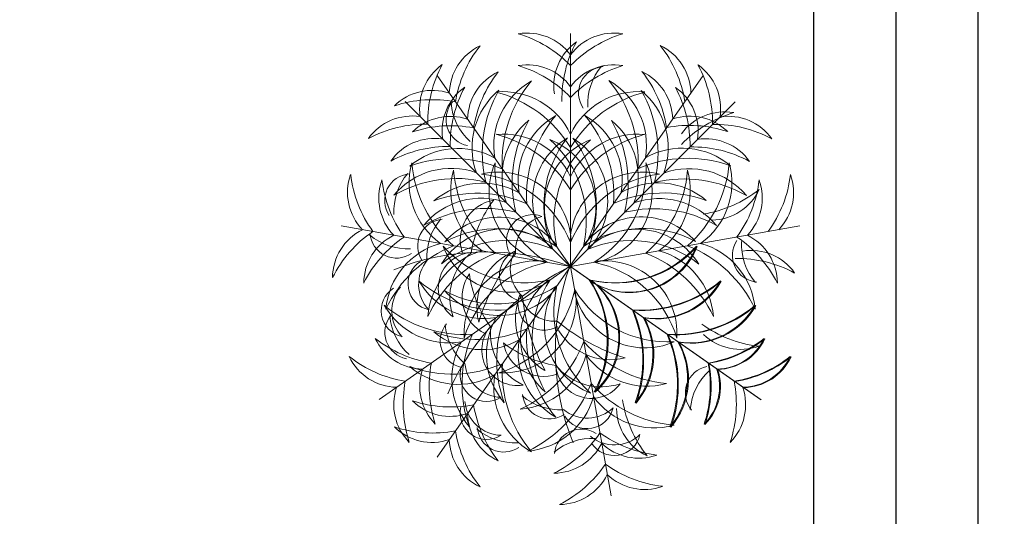
# Model space of a CAD drawing. Units: inches. Extents: x -48 to 50072, y 0 to 21068.
# Tile 38 of 75: x 501 to 555, y 279 to 306. Entities that reach past the tile are written whole.
import ezdxf

# ---------------------------------------------------------------- set-up
doc = ezdxf.new("R2010")
doc.units = ezdxf.units.IN
doc.header["$MEASUREMENT"] = 0
doc.linetypes.add('ACAD_ISO02W100', pattern=[15, 12, -3])
for name, color, linetype, lineweight in [('A-ANNO-DIMS', 2, 'Continuous', 18), ('C-PROP', 7, 'Continuous', 25), ('C-PROP-REF', 32, 'ACAD_ISO02W100', 13), ('L-PLNT', 94, 'Continuous', 13)]:
    doc.layers.add(name, color=color, linetype=linetype, lineweight=lineweight)
doc.styles.get("Standard").update_dxf_attribs({"font": 'arial.ttf'})
doc.dimstyles.get("Standard").update_dxf_attribs({"dimtxt": 8, "dimasz": 0.18, "dimexe": 0.18, "dimexo": 0.0625, "dimgap": 0.09, "dimtad": 0, "dimtih": 1, "dimtoh": 1, "dimdec": 1, "dimzin": 0, "dimdsep": 46, "dimlunit": 4, "dimtxsty": 'Standard', "dimblk": 'ARCHTICK', "dimcen": 0.09, "dimadec": 0, "dimazin": 0, "dimtfac": 1, "dimtdec": 1, "dimtofl": 0, "dimtmove": 0, "dimatfit": 3, "dimldrblk": 'ARCHTICK', "dimfxl": 1, "dimtolj": 1, "dimtzin": 0, "dimarcsym": 0})

# ---------------------------------------------------------------- blocks, each defined once
blk = doc.blocks.new('A$C5D061C3B')
for p, q in [((3.377, 6.679), (3.377, 3.377)), ((1.483, 6.082), (3.377, 3.377)), ((5.259, 6.086), (3.365, 3.381)), ((1.03, 5.716), (3.365, 3.381)), ((5.712, 5.712), (3.377, 3.377)), ((0.125, 3.951), (3.377, 3.377)), ((6.629, 3.951), (3.377, 3.377)), ((0.66, 1.487), (3.365, 3.381)), ((1.483, 0.672), (3.377, 3.377)), ((6.07, 1.487), (3.365, 3.381)), ((3.951, 0.125), (3.377, 3.377)), ((6.082, 1.483), (3.377, 3.377))]:
    blk.add_line(p, q)
for centre, radius, start, end in [((2.763, 5.924), 0.762, 36.29, 99.6243), ((2.145, 5.032), 1.715, 44.0763, 73.3794), ((3.991, 5.924), 0.762, 80.3757, 143.71), ((4.61, 5.032), 1.715, 106.6206, 135.9237), ((2.419, 5.816), 0.762, 115.3757, 178.71), ((3.438, 5.44), 1.715, 141.6206, 170.9237), ((3.901, 5.939), 0.762, 125.3757, 188.71), ((4.969, 5.745), 1.715, 151.6206, 180.9237), ((3.305, 5.444), 1.715, 9.0763, 38.3794), ((4.323, 5.82), 0.762, 1.29, 64.6243), ((1.998, 5.617), 0.762, 125.3757, 188.71), ((3.066, 5.423), 1.715, 151.6206, 180.9237), ((2.763, 5.474), 0.762, 36.29, 99.6243), ((2.145, 4.581), 1.715, 44.0763, 73.3794), ((3.991, 5.474), 0.762, 80.3757, 143.71), ((4.61, 4.581), 1.715, 106.6206, 135.9237), ((3.871, 5.832), 0.38, 94.742, 213.7475), ((4.447, 5.681), 0.826, 139.618, 183.2106), ((4.744, 5.613), 0.762, 351.29, 54.6243), ((3.676, 5.419), 1.715, 359.0763, 28.3794), ((2.678, 5.447), 0.762, 115.3757, 178.71), ((3.696, 5.07), 1.715, 141.6206, 170.9237), ((3.344, 5.089), 1.056, 119.6063, 189.7511), ((4.177, 4.869), 1.77, 139.9634, 183.6288), ((3.398, 5.094), 1.056, 350.2489, 60.3937), ((2.565, 4.873), 1.77, 356.3712, 40.0366), ((4.064, 5.451), 0.762, 1.29, 64.6243), ((3.046, 5.075), 1.715, 9.0763, 38.3794), ((1.413, 5.111), 0.762, 71.29, 134.6243), ((2.317, 5.298), 0.762, 125.3757, 188.71), ((3.385, 5.104), 1.715, 151.6206, 180.9237), ((3.035, 5.062), 1.056, 129.6063, 199.7511), ((3.894, 4.989), 1.77, 149.9634, 193.6288), ((2.848, 4.985), 1.77, 346.3712, 30.0366), ((3.707, 5.058), 1.056, 340.2489, 50.3937), ((3.357, 5.1), 1.715, 359.0763, 28.3794), ((4.425, 5.294), 0.762, 351.29, 54.6243), ((1.419, 4.026), 1.715, 79.0763, 108.3794), ((2.422, 4.799), 1.056, 25.2489, 95.3937), ((1.866, 4.14), 1.77, 31.3712, 75.0366), ((4.332, 4.799), 1.056, 84.6063, 154.7511), ((4.888, 4.14), 1.77, 104.9634, 148.6288), ((1.991, 5.462), 0.38, 139.742, 258.7475), ((2.505, 5.763), 0.826, 184.618, 228.2106), ((1.13, 4.748), 0.762, 81.29, 144.6243), ((1.671, 4.742), 0.762, 71.29, 134.6243), ((3.46, 4.637), 1.056, 129.6063, 199.7511), ((4.319, 4.565), 1.77, 149.9634, 193.6288), ((3.688, 4.597), 1.056, 119.6063, 189.7511), ((4.522, 4.377), 1.77, 139.9634, 183.6288), ((2.221, 4.381), 1.77, 356.3712, 40.0366), ((3.054, 4.602), 1.056, 350.2489, 60.3937), ((5.071, 4.746), 0.762, 45.3757, 108.71), ((5.564, 4.807), 0.762, 80.3757, 143.71), ((6.182, 3.914), 1.715, 106.6206, 135.9237), ((5.613, 4.744), 0.762, 35.3757, 98.71), ((1.324, 3.68), 1.715, 89.0763, 118.3794), ((1.677, 3.657), 1.715, 79.0763, 108.3794), ((3.283, 4.633), 1.056, 340.2489, 50.3937), ((2.424, 4.56), 1.77, 346.3712, 30.0366), ((5.065, 3.661), 1.715, 71.6206, 100.9237), ((5.419, 3.676), 1.715, 61.6206, 90.9237), ((1.448, 4.43), 0.762, 81.29, 144.6243), ((2.422, 4.198), 1.056, 25.2489, 95.3937), ((1.866, 3.54), 1.77, 31.3712, 75.0366), ((3.868, 4.321), 1.029, 121.3654, 221.5741), ((4.556, 4.237), 1.557, 141.8122, 203.3335), ((4.035, 4.215), 1.029, 111.3654, 211.5741), ((2.707, 4.219), 1.029, 328.4259, 68.6346), ((2.044, 4.017), 1.557, 346.6665, 48.1878), ((4.698, 4.013), 1.557, 131.8122, 193.3335), ((4.332, 4.198), 1.056, 84.6063, 154.7511), ((4.888, 3.54), 1.77, 104.9634, 148.6288), ((2.187, 4.233), 1.557, 336.6665, 38.1878), ((2.875, 4.316), 1.029, 318.4259, 58.6346), ((5.294, 4.425), 0.762, 35.3757, 98.71), ((1.642, 3.362), 1.715, 89.0763, 118.3794), ((1.78, 3.994), 1.056, 60.2489, 130.3937), ((4.963, 3.998), 1.056, 49.6063, 119.7511), ((5.1, 3.357), 1.715, 61.6206, 90.9237), ((1.702, 3.136), 1.77, 66.3712, 110.0366), ((5.04, 3.14), 1.77, 69.9634, 113.6288), ((1.685, 3.712), 1.056, 70.2489, 140.3937), ((2.143, 4.564), 1.056, 164.6063, 234.7511), ((2.888, 4.998), 1.77, 184.9634, 228.6288), ((3.25, 4.435), 1.029, 156.3654, 256.5741), ((3.862, 4.761), 1.557, 176.8122, 238.3335), ((2.893, 4.761), 1.557, 301.6665, 3.1878), ((3.504, 4.435), 1.029, 283.4259, 23.6346), ((5.058, 3.707), 1.056, 39.6063, 109.7511), ((3.866, 4.998), 1.77, 311.3712, 355.0366), ((4.611, 4.564), 1.056, 305.2489, 15.3937), ((0.975, 4.424), 0.762, 160.3757, 223.71), ((1.962, 4.878), 1.715, 186.6206, 215.9237), ((1.12, 4.31), 0.38, 94.742, 213.7475), ((1.696, 4.159), 0.826, 139.618, 183.2106), ((1.757, 2.853), 1.77, 76.3712, 120.0366), ((2.734, 4.46), 1.056, 164.6063, 234.7511), ((3.48, 4.893), 1.77, 184.9634, 228.6288), ((2.358, 3.686), 1.029, 3.4259, 103.6346), ((1.93, 3.14), 1.557, 21.6665, 83.1878), ((4.397, 3.686), 1.029, 76.3654, 176.5741), ((4.824, 3.14), 1.557, 96.8122, 158.3335), ((3.275, 4.893), 1.77, 311.3712, 355.0366), ((4.985, 2.848), 1.77, 59.9634, 103.6288), ((4.02, 4.46), 1.056, 305.2489, 15.3937), ((4.793, 4.878), 1.715, 324.0763, 353.3794), ((5.779, 4.424), 0.762, 316.29, 19.6243), ((1.419, 4.346), 0.762, 160.3757, 223.71), ((2.405, 4.8), 1.715, 186.6206, 215.9237), ((2.124, 3.502), 1.056, 60.2489, 130.3937), ((4.618, 3.506), 1.056, 49.6063, 119.7511), ((4.349, 4.8), 1.715, 324.0763, 353.3794), ((5.335, 4.346), 0.762, 316.29, 19.6243), ((2.109, 3.287), 1.056, 70.2489, 140.3937), ((2.046, 2.644), 1.77, 66.3712, 110.0366), ((4.696, 2.648), 1.77, 69.9634, 113.6288), ((4.633, 3.283), 1.056, 39.6063, 109.7511), ((4.988, 5.812), 1.715, 279.0763, 308.3794), ((5.365, 4.794), 0.762, 271.29, 334.6243), ((2.182, 2.428), 1.77, 76.3712, 120.0366), ((2.387, 3.752), 0.574, 99.9865, 199.4034), ((3.599, 3.314), 1.651, 142.5759, 170.8942), ((4.56, 2.424), 1.77, 59.9634, 103.6288), ((2.365, 3.045), 1.029, 38.4259, 138.6346), ((2.84, 3.739), 0.372, 69.2257, 210.1279), ((3.109, 3.59), 0.515, 105.4398, 183.6694), ((4.377, 3.05), 1.029, 41.3654, 141.5741), ((1.588, 3.666), 0.38, 94.742, 213.7475), ((2.165, 3.515), 0.826, 139.618, 183.2106), ((4.414, 2.358), 1.557, 61.8122, 123.3335), ((0.762, 3.214), 0.762, 116.29, 179.6243), ((1.534, 2.451), 1.715, 124.0763, 153.3794), ((1.206, 3.136), 0.762, 116.29, 179.6243), ((1.977, 2.373), 1.715, 124.0763, 153.3794), ((1.062, 4.452), 0.826, 229.618, 273.2106), ((0.91, 3.875), 0.38, 184.742, 303.7475), ((2.426, 2.879), 1.029, 48.4259, 148.6346), ((2.328, 2.353), 1.557, 56.6665, 118.1878), ((4.316, 2.875), 1.029, 31.3654, 131.5741), ((4.777, 2.373), 1.715, 26.6206, 55.9237), ((5.549, 3.136), 0.762, 0.3757, 63.71), ((1.811, 2.684), 1.056, 105.2489, 175.3937), ((2.363, 2.022), 1.77, 111.3712, 155.0366), ((2.51, 2.191), 1.557, 66.6665, 128.1878), ((2.729, 4.702), 1.557, 221.8122, 283.3335), ((2.527, 4.039), 1.029, 201.3654, 301.5741), ((4.233, 2.187), 1.557, 51.8122, 113.3335), ((4.001, 4.702), 1.557, 256.6665, 318.1878), ((4.013, 4.698), 1.557, 256.6665, 318.1878), ((4.203, 4.039), 1.029, 238.4259, 338.6346), ((4.215, 4.035), 1.029, 238.4259, 338.6346), ((4.391, 2.022), 1.77, 24.9634, 68.6288), ((4.943, 2.684), 1.056, 4.6063, 74.7511), ((6.053, 3.533), 0.38, 146.2525, 265.258), ((6.629, 3.684), 0.826, 176.7894, 220.382), ((2.185, 0.015), 3.567, 70.4772, 111.6585), ((2.403, 2.58), 1.056, 105.2489, 175.3937), ((2.955, 1.917), 1.77, 111.3712, 155.0366), ((2.007, 3.071), 0.506, 93.8744, 233.9763), ((2.489, 2.932), 0.825, 128.7536, 199.097), ((2.903, 2.8), 0.855, 116.4477, 194.3672), ((4.744, 1.779), 2.789, 140.4007, 163.139), ((2.741, 3.253), 0.372, 114.2257, 255.1279), ((3.037, 3.338), 0.515, 150.4398, 228.6694), ((3.799, 1.917), 1.77, 24.9634, 68.6288), ((4.352, 2.58), 1.056, 4.6063, 74.7511), ((5.935, 2.842), 0.762, 35.3757, 98.71), ((1.447, 3.129), 0.376, 122.0577, 257.8533), ((1.751, 3.126), 0.529, 140.1845, 223.654), ((4.912, 0.157), 3.567, 115.4772, 156.6585), ((2.896, 2.427), 1.029, 83.4259, 183.6346), ((3.359, 1.911), 1.557, 101.6665, 163.1878), ((6.727, 2.189), 3.567, 160.4772, 201.6585), ((3.395, 1.911), 1.557, 16.8122, 78.3335), ((3.858, 2.427), 1.029, 356.3654, 96.5741), ((5.741, 1.774), 1.715, 61.6206, 90.9237), ((2.412, 2.943), 0.574, 144.9865, 244.4034), ((3.578, 3.49), 1.651, 187.5759, 215.8942), ((1.37, 2.745), 0.529, 140.1845, 223.654), ((2.145, 3.693), 1.056, 209.6063, 279.7511), ((2.365, 4.526), 1.77, 229.9634, 273.6288), ((2.328, 4.401), 1.557, 241.8122, 303.3335), ((3.697, 2.369), 1.029, 128.4259, 228.6346), ((4.389, 2.332), 1.557, 146.6665, 208.1878), ((4.035, 2.539), 1.029, 148.4259, 248.6346), ((4.698, 2.741), 1.557, 166.6665, 228.1878), ((2.341, 2.332), 1.557, 331.8122, 33.3335), ((2.353, 2.328), 1.557, 331.8122, 33.3335), ((3.033, 2.369), 1.029, 311.3654, 51.5741), ((3.045, 2.365), 1.029, 311.3654, 51.5741), ((4.365, 4.526), 1.77, 266.3712, 310.0366), ((4.377, 4.522), 1.77, 266.3712, 310.0366), ((4.585, 3.693), 1.056, 260.2489, 330.3937), ((4.597, 3.688), 1.056, 260.2489, 330.3937), ((1.067, 2.749), 0.376, 122.0577, 257.8533), ((2.365, 3.709), 1.029, 221.3654, 321.5741), ((1.911, 3.359), 1.557, 286.8122, 348.3335), ((2.427, 2.896), 1.029, 266.3654, 6.5741), ((3.003, 2.844), 0.372, 159.2257, 300.1279), ((3.152, 3.113), 0.515, 195.4398, 273.6694), ((5.474, 3.214), 2.789, 185.4007, 208.139), ((4.435, 3.25), 1.029, 193.4259, 293.6346), ((4.761, 3.862), 1.557, 211.6665, 273.1878), ((1.873, 4.181), 1.77, 229.9634, 273.6288), ((1.653, 3.348), 1.056, 209.6063, 279.7511), ((3.45, 2.634), 0.855, 161.4477, 239.3672), ((4.857, 4.181), 1.77, 266.3712, 310.0366), ((4.869, 4.177), 1.77, 266.3712, 310.0366), ((5.077, 3.348), 1.056, 260.2489, 330.3937), ((5.089, 3.344), 1.056, 260.2489, 330.3937), ((1.122, 2.441), 0.38, 139.742, 258.7475), ((1.636, 2.741), 0.826, 184.618, 228.2106), ((4.099, 2.051), 1.77, 156.3712, 200.0366), ((2.632, 2.051), 1.77, 339.9634, 23.6288), ((2.644, 2.046), 1.77, 339.9634, 23.6288), ((1.908, 2.317), 0.38, 139.742, 258.7475), ((2.422, 2.617), 0.826, 184.618, 228.2106), ((2.624, 2.192), 0.506, 138.8744, 278.9763), ((3.24, 2.128), 1.056, 150.2489, 220.3937), ((3.064, 2.435), 0.825, 173.7536, 244.097), ((3.942, 2.908), 0.855, 206.4477, 284.3672), ((4.963, 4.749), 2.789, 230.4007, 253.139), ((3.49, 2.128), 1.056, 319.6063, 29.7511), ((3.502, 2.124), 1.056, 319.6063, 29.7511), ((6.244, 3.948), 1.715, 234.0763, 263.3794), ((2.046, 4.111), 1.77, 249.9634, 293.6288), ((2.124, 3.252), 1.056, 229.6063, 299.7511), ((3.607, 1.706), 1.77, 156.3712, 200.0366), ((4.522, 2.378), 1.77, 176.3712, 220.0366), ((3.124, 1.706), 1.77, 339.9634, 23.6288), ((3.136, 1.702), 1.77, 339.9634, 23.6288), ((5.79, 2.962), 0.762, 226.29, 289.6243), ((1.672, 3.7), 1.715, 231.6206, 260.9237), ((1.295, 2.682), 0.762, 205.3757, 268.71), ((2.748, 1.784), 1.056, 150.2489, 220.3937), ((3.428, 3.603), 1.651, 232.5759, 260.8942), ((2.99, 2.391), 0.574, 189.9865, 289.4034), ((3.688, 2.157), 1.056, 170.2489, 240.3937), ((1.917, 2.955), 1.77, 294.9634, 338.6288), ((4.893, 3.48), 1.77, 221.3712, 265.0366), ((3.982, 1.784), 1.056, 319.6063, 29.7511), ((3.994, 1.78), 1.056, 319.6063, 29.7511), ((5.058, 3.7), 1.715, 279.0763, 308.3794), ((5.07, 3.696), 1.715, 279.0763, 308.3794), ((5.435, 2.682), 0.762, 271.29, 334.6243), ((5.447, 2.678), 0.762, 271.29, 334.6243), ((0.926, 2.424), 0.762, 205.3757, 268.71), ((1.303, 3.442), 1.715, 231.6206, 260.9237), ((2.58, 2.403), 1.056, 274.6063, 344.7511), ((4.46, 2.734), 1.056, 215.2489, 285.3937), ((5.427, 3.442), 1.715, 279.0763, 308.3794), ((5.804, 2.424), 0.762, 271.29, 334.6243), ((1.702, 3.619), 1.77, 249.9634, 293.6288), ((1.78, 2.76), 1.056, 229.6063, 299.7511), ((3.086, 1.681), 1.715, 169.0763, 198.3794), ((2.405, 2.049), 0.529, 185.1845, 268.654), ((4.177, 1.886), 1.77, 176.3712, 220.0366), ((3.81, 2.493), 0.825, 218.7536, 289.097), ((3.671, 2.011), 0.506, 183.8744, 323.9763), ((5.385, 1.584), 0.38, 101.2525, 220.258), ((3.645, 1.681), 1.715, 341.6206, 10.9237), ((3.657, 1.677), 1.715, 341.6206, 10.9237), ((5.44, 3.438), 1.715, 279.0763, 308.3794), ((5.816, 2.419), 0.762, 271.29, 334.6243), ((2, 1.676), 0.762, 161.29, 224.6243), ((2.188, 1.837), 0.376, 167.0577, 302.8533), ((3.344, 1.665), 1.056, 170.2489, 240.3937), ((5.899, 1.283), 0.826, 131.7894, 175.382), ((4.73, 1.676), 0.762, 315.3757, 18.71), ((4.742, 1.671), 0.762, 315.3757, 18.71), ((2.717, 1.423), 1.715, 169.0763, 198.3794), ((2.022, 2.363), 1.77, 294.9634, 338.6288), ((4.998, 2.888), 1.77, 221.3712, 265.0366), ((4.014, 1.423), 1.715, 341.6206, 10.9237), ((1.631, 1.417), 0.762, 161.29, 224.6243), ((3.227, 2.169), 0.826, 229.618, 273.2106), ((3.076, 1.593), 0.38, 184.742, 303.7475), ((5.099, 1.417), 0.762, 315.3757, 18.71), ((1.671, 2.012), 0.762, 225.3757, 288.71), ((1.677, 3.098), 1.715, 251.6206, 280.9237), ((2.405, 1.511), 0.529, 185.1845, 268.654), ((3.696, 1.684), 1.715, 189.0763, 218.3794), ((2.684, 1.811), 1.056, 274.6063, 344.7511), ((4.564, 2.143), 1.056, 215.2489, 285.3937), ((5.808, 1.754), 1.715, 189.0763, 218.3794), ((2.188, 1.299), 0.376, 167.0577, 302.8533), ((2.678, 1.307), 0.762, 181.29, 244.6243), ((3.616, 1.755), 0.529, 230.1845, 313.654), ((3.613, 1.452), 0.376, 212.0577, 347.8533), ((4.79, 1.377), 0.762, 181.29, 244.6243), ((1.419, 2.729), 1.715, 251.6206, 280.9237), ((1.413, 1.643), 0.762, 225.3757, 288.71), ((3.438, 1.315), 1.715, 189.0763, 218.3794), ((2.583, 1.701), 0.826, 229.618, 273.2106), ((2.432, 1.124), 0.38, 184.742, 303.7475), ((2.373, 1.977), 1.715, 296.6206, 325.9237), ((3.528, 0.69), 0.38, 56.2525, 175.258), ((3.997, 1.374), 0.529, 230.1845, 313.654), ((3.994, 1.071), 0.376, 212.0577, 347.8533), ((4.8, 2.405), 1.715, 234.0763, 263.3794), ((2.419, 0.938), 0.762, 181.29, 244.6243), ((3.136, 1.206), 0.762, 270.3757, 333.71), ((3.68, 0.113), 0.826, 86.7894, 130.382), ((4.346, 1.419), 0.762, 226.29, 289.6243), ((2.451, 1.534), 1.715, 296.6206, 325.9237), ((4.878, 1.962), 1.715, 234.0763, 263.3794), ((3.214, 0.762), 0.762, 270.3757, 333.71), ((4.424, 0.975), 0.762, 226.29, 289.6243)]:
    blk.add_arc(centre, radius, start, end)
blk = doc.blocks.new('_ArchTick')
at = {"color": 0, "linetype": 'ByBlock', "const_width": 0.15}
blk.add_lwpolyline([(-0.5, -0.5), (0.5, 0.5)], dxfattribs=at)
blk = doc.blocks.new('*D54')
at = {"layer": 'A-ANNO-DIMS', "color": 0, "lineweight": -2, "transparency": 16777216}
for p, q in [((540.551, 275.597), (544.198, 275.597)), ((544.018, 275.597), (544.018, 268.06)), ((544.018, 252.07), (544.018, 259.607)), ((540.551, 252.07), (544.198, 252.07))]:
    blk.add_line(p, q, dxfattribs=at)
at = {"layer": 'Defpoints', "color": 0, "transparency": 16777216}
for p in [(540.489, 275.597), (544.018, 275.597), (540.489, 252.07)]:
    blk.add_point(p, dxfattribs=at)
at = {"layer": 'A-ANNO-DIMS', "color": 0, "lineweight": -2, "transparency": 16777216, "xscale": 0.18, "yscale": 0.18, "zscale": 0.18}
for p, rotation in [((544.018, 275.597), 90), ((544.018, 252.07), 270)]:
    blk.add_blockref('_ArchTick', p, dxfattribs=dict(at, rotation=rotation))
at = {"layer": 'A-ANNO-DIMS', "color": 0, "transparency": 16777216, "insert": (544.018, 263.834), "char_height": 8, "attachment_point": 5}
blk.add_mtext('\\A1;SHRUB B 24 TYP.', dxfattribs=at)
blk = doc.blocks.new('*D115')
at = {"layer": 'A-ANNO-DIMS', "color": 0, "lineweight": -2, "transparency": 16777216}
for p, q in [((549.08, 451.075), (601.647, 451.075)), ((601.467, 451.075), (601.467, 336.752)), ((601.467, 214.075), (601.467, 328.397)), ((553.58, 214.075), (601.647, 214.075))]:
    blk.add_line(p, q, dxfattribs=at)
at = {"layer": 'Defpoints', "color": 0, "transparency": 16777216}
for p in [(549.017, 451.075), (601.467, 451.075), (553.517, 214.075)]:
    blk.add_point(p, dxfattribs=at)
at = {"layer": 'A-ANNO-DIMS', "color": 0, "lineweight": -2, "transparency": 16777216, "xscale": 0.18, "yscale": 0.18, "zscale": 0.18}
for p, rotation in [((601.467, 451.075), 90), ((601.467, 214.075), 270)]:
    blk.add_blockref('_ArchTick', p, dxfattribs=dict(at, rotation=rotation))
at = {"layer": 'A-ANNO-DIMS', "color": 0, "transparency": 16777216, "insert": (601.467, 332.575), "char_height": 8, "attachment_point": 5}
blk.add_mtext('\\A1;237', dxfattribs=at)
blk = doc.blocks.new('*D119')
at = {"layer": 'A-ANNO-DIMS', "color": 0, "lineweight": -2, "transparency": 16777216}
for p, q in [((463.517, 451.012), (463.517, 165.945)), ((549.017, 451.012), (549.017, 165.945)), ((463.517, 166.125), (495.752, 166.125)), ((549.017, 166.125), (516.783, 166.125))]:
    blk.add_line(p, q, dxfattribs=at)
at = {"layer": 'Defpoints', "color": 0, "transparency": 16777216}
for p in [(463.517, 451.075), (549.017, 451.075), (549.017, 166.125)]:
    blk.add_point(p, dxfattribs=at)
at = {"layer": 'A-ANNO-DIMS', "color": 0, "lineweight": -2, "transparency": 16777216, "xscale": 0.18, "yscale": 0.18, "zscale": 0.18, "rotation": 180}
blk.add_blockref('_ArchTick', (463.517, 166.125), dxfattribs=at)
at = {"layer": 'A-ANNO-DIMS', "color": 0, "lineweight": -2, "transparency": 16777216, "xscale": 0.18, "yscale": 0.18, "zscale": 0.18}
blk.add_blockref('_ArchTick', (549.017, 166.125), dxfattribs=at)
at = {"layer": 'A-ANNO-DIMS', "color": 0, "transparency": 16777216, "insert": (506.267, 166.125), "char_height": 8, "attachment_point": 5}
blk.add_mtext('\\A1;85.5', dxfattribs=at)

msp = doc.modelspace()

# ---------------------------------------------------------------- linework, layer by layer
at = {"layer": 'C-PROP'}
for p, q in [((553.517, 214.075), (553.517, 1170.775)), ((544.517, 223.075), (544.517, 488.775))]:
    msp.add_line(p, q, dxfattribs=at)
at = {"layer": 'C-PROP-REF'}
msp.add_line((549.017, 214.075), (549.017, 1166.275), dxfattribs=at)

# ---------------------------------------------------------------- block references
at = {"layer": 'L-PLNT', "xscale": 3.862191520948588, "yscale": 3.862191520948588, "zscale": 3.862191520948588}
msp.add_blockref('A$C5D061C3B', (518.144, 279.329), dxfattribs=at)

# ---------------------------------------------------------------- dimensions: what is measured, and where the dimension line sits
at = {"layer": 'A-ANNO-DIMS'}
dim = msp.add_linear_dim(base=(549.017, 166.125), p1=(463.517, 451.075), p2=(549.017, 451.075), dimstyle='Standard', override={"dimdec": 1, "dimlfac": 1, "dimrnd": 0, "dimzin": 0, "dimdsep": 46, "dimlunit": 2}, dxfattribs=at)
dim.commit()
dim.dimension.update_dxf_attribs({"geometry": '*D119', "text_midpoint": (506.267, 166.125)})
dim = msp.add_linear_dim(base=(601.467, 451.075), p1=(553.517, 214.075), p2=(549.017, 451.075), angle=90, dimstyle='Standard', override={"dimdec": 0, "dimlfac": 1, "dimrnd": 0, "dimzin": 0, "dimdsep": 46, "dimlunit": 2}, dxfattribs=at)
dim.commit()
dim.dimension.update_dxf_attribs({"geometry": '*D115', "text_midpoint": (601.467, 332.575)})
dim = msp.add_linear_dim(base=(544.018, 275.597), p1=(540.489, 252.07), p2=(540.489, 275.597), angle=90, text='SHRUB B <> TYP.', dimstyle='Standard', override={"dimdec": 0, "dimlfac": 1, "dimrnd": 0, "dimzin": 0, "dimdsep": 46, "dimlunit": 2}, dxfattribs=at)
dim.commit()
dim.dimension.update_dxf_attribs({"geometry": '*D54', "text_midpoint": (544.018, 263.834)})

doc.saveas('drawing.dxf')
